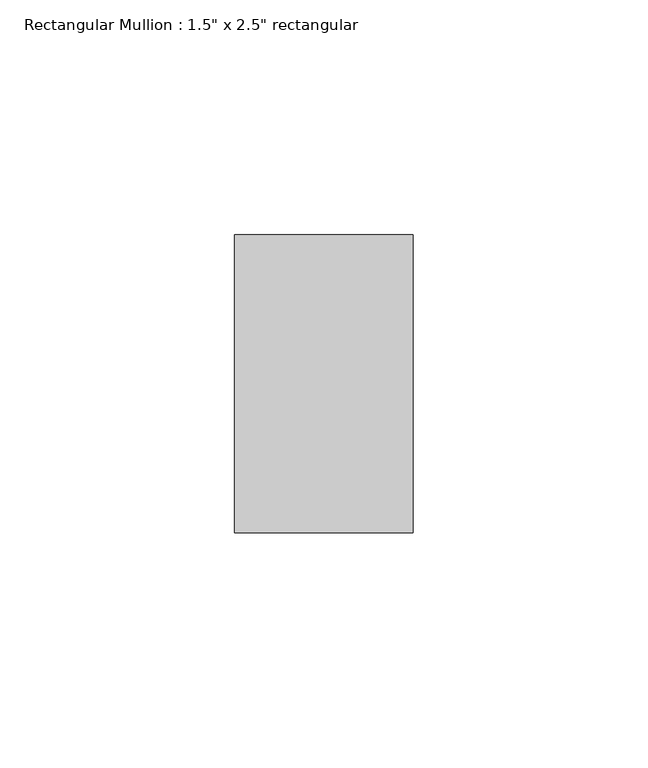
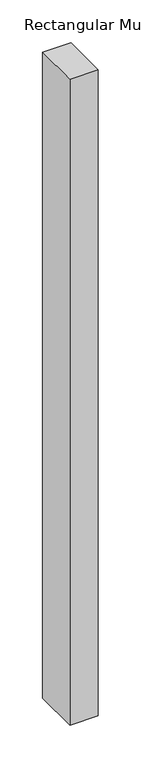
"""IFC4 building model written with IfcOpenShell, lengths in millimetres: member geometry."""

from ifc_helpers import new_model, si_unit, frame, origin, place, context, project, spatial, polyline, outline, extrude, source, transform, mapped, element, save


def member_c9b54d35(model_context):
    return source(origin(), model_context, "Body", "SweptSolid", [
        extrude(outline(polyline([(19.05, 31.75), (19.05, -31.75), (-19.05, -31.75), (-19.05, 31.75), (19.05, 31.75)])), frame((0.0, 0.0, -920.75), z_axis=(0.0, 0.0, 1.0), x_axis=(1.0, 0.0, 0.0)), (0.0, 0.0, 1.0), 920.75),
    ])


if __name__ == "__main__":
    model = new_model("IFC4")
    model_context = context("Model", 3, world=origin())
    ifc_project = project(units=[si_unit("LENGTHUNIT", "METRE", prefix="MILLI")], contexts=[model_context])
    site = spatial("IfcSite", under=ifc_project)
    building = spatial("IfcBuilding", under=site)
    placement = place(None, origin())
    member_shape = member_c9b54d35(model_context)
    element("IfcMember", 1, ObjectType="Rectangular Mullion : 1.5\" x 2.5\" rectangular", at=placement, inside=building, context=model_context, shape_type="MappedRepresentation", body=[
        mapped(member_shape, transform((0.0, 0.0, 0.0), x_axis=(1.0, 0.0, 0.0), y_axis=(0.0, 1.0, 0.0), z_axis=(0.0, 0.0, 1.0))),
    ])
    save(model, "model.ifc")

# Revit data of these elements
# Type "Rectangular Mullion : 1.5\" x 2.5\" rectangular"
#   built-in parameter 1007304 = 0.208333 (stored number, unit not read)
#   built-in parameter 1007301 = 0.0625 (stored number, unit not read)
#   built-in parameter 1007300 = 0.0625 (stored number, unit not read)
